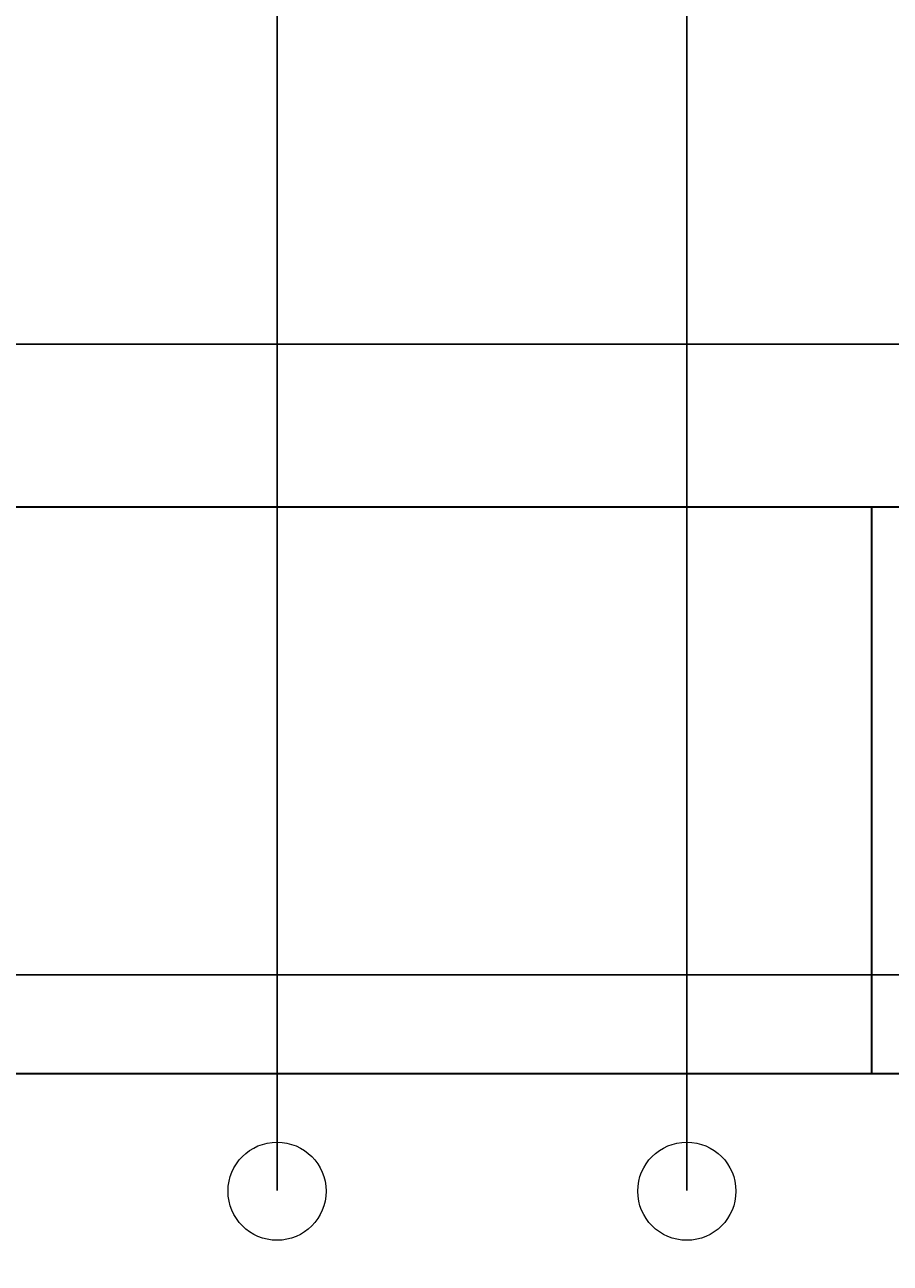
# Model space of a CAD drawing. Units: inches. Extents: x -13 to 809, y 112 to 656.
# Tile 30 of 55: x 183 to 257, y 446 to 551. Entities that reach past the tile are written whole.
import ezdxf

# ---------------------------------------------------------------- set-up
doc = ezdxf.new("R2010")
doc.units = ezdxf.units.IN
doc.header["$MEASUREMENT"] = 0
for name, color, linetype, lineweight in [('A-ANNO-DIMS', 2, 'Continuous', 18), ('A-ELEV', 7, 'Continuous', 35), ('A-ELEV-OTLN', 7, 'Continuous', 18)]:
    doc.layers.add(name, color=color, linetype=linetype, lineweight=lineweight)
doc.styles.get("Standard").update_dxf_attribs({"font": 'arial.ttf'})
doc.dimstyles.get("Standard").update_dxf_attribs({"dimtxt": 0.625, "dimasz": 0.18, "dimexe": 0.18, "dimexo": 0.0625, "dimgap": 0.09, "dimtad": 0, "dimtih": 1, "dimtoh": 1, "dimdec": 4, "dimzin": 0, "dimdsep": 46, "dimlunit": 4, "dimtxsty": 'Standard', "dimcen": 0.09, "dimadec": 0, "dimazin": 0, "dimtfac": 1, "dimtdec": 4, "dimtofl": 0, "dimtmove": 0, "dimatfit": 3, "dimfxl": 1, "dimtolj": 1, "dimtzin": 0, "dimarcsym": 0})

# ---------------------------------------------------------------- blocks, each defined once
blk = doc.blocks.new('*D23')
at = {"layer": 'A-ANNO-DIMS', "color": 0, "lineweight": -2, "transparency": 16777216}
for p, q in [((107.26, 510.58), (107.26, 655.96)), ((107.44, 655.78), (198.73, 655.78)), ((292.74, 655.78), (201.45, 655.78)), ((292.92, 569.3), (292.92, 655.96))]:
    blk.add_line(p, q, dxfattribs=at)
at = {"layer": 'A-ANNO-DIMS', "color": 0, "transparency": 16777216}
for points in [[(107.44, 655.81), (107.44, 655.75), (107.26, 655.78)], [(292.74, 655.81), (292.74, 655.75), (292.92, 655.78)]]:
    blk.add_solid(points, dxfattribs=at)
at = {"layer": 'Defpoints', "color": 0, "transparency": 16777216}
for p in [(292.92, 655.78), (292.92, 569.24), (107.26, 510.52)]:
    blk.add_point(p, dxfattribs=at)
at = {"layer": 'A-ANNO-DIMS', "color": 0, "transparency": 16777216, "insert": (200.09, 655.78), "char_height": 0.625, "attachment_point": 5}
blk.add_mtext('\\A1;185.66', dxfattribs=at)
blk = doc.blocks.new('*D36')
at = {"layer": 'A-ANNO-DIMS', "color": 0, "lineweight": -2, "transparency": 16777216}
for p, q in [((311.64, 569.24), (-12.1, 569.24)), ((-11.92, 569.06), (-11.92, 540.29)), ((-11.92, 510.7), (-11.92, 539.47)), ((107.2, 510.52), (-12.1, 510.52))]:
    blk.add_line(p, q, dxfattribs=at)
at = {"layer": 'A-ANNO-DIMS', "color": 0, "transparency": 16777216}
for points in [[(-11.95, 569.06), (-11.89, 569.06), (-11.92, 569.24)], [(-11.95, 510.7), (-11.89, 510.7), (-11.92, 510.52)]]:
    blk.add_solid(points, dxfattribs=at)
at = {"layer": 'Defpoints', "color": 0, "transparency": 16777216}
for p in [(-11.92, 569.24), (311.7, 569.24), (107.26, 510.52)]:
    blk.add_point(p, dxfattribs=at)
at = {"layer": 'A-ANNO-DIMS', "color": 0, "transparency": 16777216, "insert": (-11.92, 539.88), "char_height": 0.625, "attachment_point": 5}
blk.add_mtext('\\A1;58.72', dxfattribs=at)
blk = doc.blocks.new('*D39')
at = {"layer": 'A-ANNO-DIMS', "color": 0, "lineweight": -2, "transparency": 16777216}
for p, q in [((341.34, 524.28), (-12.1, 524.28)), ((-11.92, 524.1), (-11.92, 406.78)), ((-11.92, 288.63), (-11.92, 405.96)), ((341.34, 288.45), (-12.1, 288.45))]:
    blk.add_line(p, q, dxfattribs=at)
at = {"layer": 'A-ANNO-DIMS', "color": 0, "transparency": 16777216}
for points in [[(-11.95, 524.1), (-11.89, 524.1), (-11.92, 524.28)], [(-11.95, 288.63), (-11.89, 288.63), (-11.92, 288.45)]]:
    blk.add_solid(points, dxfattribs=at)
at = {"layer": 'Defpoints', "color": 0, "transparency": 16777216}
for p in [(-11.92, 524.28), (341.41, 524.28), (341.41, 288.45)]:
    blk.add_point(p, dxfattribs=at)
at = {"layer": 'A-ANNO-DIMS', "color": 0, "transparency": 16777216, "insert": (-11.92, 406.37), "char_height": 0.625, "attachment_point": 5}
blk.add_mtext('\\A1;235.83', dxfattribs=at)
blk = doc.blocks.new('*D43')
at = {"layer": 'A-ANNO-DIMS', "color": 0, "lineweight": -2, "transparency": 16777216}
for p, q in [((471.04, 470.88), (-12.1, 470.88)), ((-11.92, 470.7), (-11.92, 443.28)), ((-11.92, 415.04), (-11.92, 442.46)), ((471.04, 414.86), (-12.1, 414.86))]:
    blk.add_line(p, q, dxfattribs=at)
at = {"layer": 'A-ANNO-DIMS', "color": 0, "transparency": 16777216}
for points in [[(-11.95, 470.7), (-11.89, 470.7), (-11.92, 470.88)], [(-11.95, 415.04), (-11.89, 415.04), (-11.92, 414.86)]]:
    blk.add_solid(points, dxfattribs=at)
at = {"layer": 'Defpoints', "color": 0, "transparency": 16777216}
for p in [(-11.92, 470.88), (471.1, 470.88), (471.1, 414.86)]:
    blk.add_point(p, dxfattribs=at)
at = {"layer": 'A-ANNO-DIMS', "color": 0, "transparency": 16777216, "insert": (-11.92, 442.87), "char_height": 0.625, "attachment_point": 5}
blk.add_mtext('\\A1;56.02', dxfattribs=at)
blk = doc.blocks.new('*D98')
at = {"layer": 'A-ANNO-DIMS', "color": 0, "lineweight": -2, "transparency": 16777216}
for p, q in [((177.59, 452.63), (177.59, 655.96)), ((177.77, 655.78), (189.7, 655.78)), ((204.42, 655.78), (192.49, 655.78)), ((204.6, 452.63), (204.6, 655.96))]:
    blk.add_line(p, q, dxfattribs=at)
at = {"layer": 'A-ANNO-DIMS', "color": 0, "transparency": 16777216}
for points in [[(177.77, 655.81), (177.77, 655.75), (177.59, 655.78)], [(204.42, 655.81), (204.42, 655.75), (204.6, 655.78)]]:
    blk.add_solid(points, dxfattribs=at)
at = {"layer": 'Defpoints', "color": 0, "transparency": 16777216}
for p in [(204.6, 655.78), (177.59, 452.56), (204.6, 452.56)]:
    blk.add_point(p, dxfattribs=at)
at = {"layer": 'A-ANNO-DIMS', "color": 0, "transparency": 16777216, "insert": (191.09, 655.78), "char_height": 0.625, "attachment_point": 5}
blk.add_mtext('\\A1;27.017', dxfattribs=at)
blk = doc.blocks.new('*D99')
at = {"layer": 'A-ANNO-DIMS', "color": 0, "lineweight": -2, "transparency": 16777216}
for p, q in [((204.6, 452.63), (204.6, 655.96)), ((204.78, 655.78), (220.57, 655.78)), ((239.13, 655.78), (223.34, 655.78)), ((239.31, 452.63), (239.31, 655.96))]:
    blk.add_line(p, q, dxfattribs=at)
at = {"layer": 'A-ANNO-DIMS', "color": 0, "transparency": 16777216}
for points in [[(204.78, 655.81), (204.78, 655.75), (204.6, 655.78)], [(239.13, 655.81), (239.13, 655.75), (239.31, 655.78)]]:
    blk.add_solid(points, dxfattribs=at)
at = {"layer": 'Defpoints', "color": 0, "transparency": 16777216}
for p in [(239.31, 655.78), (204.6, 452.56), (239.31, 452.56)]:
    blk.add_point(p, dxfattribs=at)
at = {"layer": 'A-ANNO-DIMS', "color": 0, "transparency": 16777216, "insert": (221.96, 655.78), "char_height": 0.625, "attachment_point": 5}
blk.add_mtext('\\A1;34.705', dxfattribs=at)
blk = doc.blocks.new('*D100')
at = {"layer": 'A-ANNO-DIMS', "color": 0, "lineweight": -2, "transparency": 16777216}
for p, q in [((239.31, 452.63), (239.31, 655.96)), ((239.49, 655.78), (252.41, 655.78)), ((268.12, 655.78), (255.2, 655.78)), ((268.3, 452.63), (268.3, 655.96))]:
    blk.add_line(p, q, dxfattribs=at)
at = {"layer": 'A-ANNO-DIMS', "color": 0, "transparency": 16777216}
for points in [[(239.49, 655.81), (239.49, 655.75), (239.31, 655.78)], [(268.12, 655.81), (268.12, 655.75), (268.3, 655.78)]]:
    blk.add_solid(points, dxfattribs=at)
at = {"layer": 'Defpoints', "color": 0, "transparency": 16777216}
for p in [(268.3, 655.78), (239.31, 452.56), (268.3, 452.56)]:
    blk.add_point(p, dxfattribs=at)
at = {"layer": 'A-ANNO-DIMS', "color": 0, "transparency": 16777216, "insert": (253.8, 655.78), "char_height": 0.625, "attachment_point": 5}
blk.add_mtext('\\A1;28.994', dxfattribs=at)

msp = doc.modelspace()

# ---------------------------------------------------------------- linework, layer by layer
at = {"layer": 'A-ELEV'}
for p, q in [((107.2588, 510.5199), (341.4072, 510.5199)), ((254.968, 462.5199), (254.968, 510.5199)), ((95.0469, 462.5199), (337.5074, 462.5199))]:
    msp.add_line(p, q, dxfattribs=at)
at = {"layer": 'A-ELEV-OTLN'}
for centre in [(204.6029, 452.5629), (239.3079, 452.5629)]:
    msp.add_circle(centre, 4.1542, dxfattribs=at)

# ---------------------------------------------------------------- dimensions: what is measured, and where the dimension line sits
at = {"layer": 'A-ANNO-DIMS'}
for base, p1, p2, override, picture, middle in [((292.923, 655.7828), (107.2588, 510.5199), (292.923, 569.2414), {"dimdec": 2, "dimlfac": 1, "dimrnd": 0, "dimzin": 0, "dimdsep": 46, "dimlunit": 2}, '*D23', (200.0909, 655.7828)), ((204.6029, 655.7828), (177.5857, 452.5629), (204.6029, 452.5629), {"dimdec": 3, "dimlfac": 1, "dimrnd": 0, "dimzin": 0, "dimdsep": 46, "dimlunit": 2}, '*D98', (191.0943, 655.7828)), ((239.3079, 655.7828), (204.6029, 452.5629), (239.3079, 452.5629), {"dimdec": 3, "dimlfac": 1, "dimrnd": 0, "dimzin": 0, "dimdsep": 46, "dimlunit": 2}, '*D99', (221.9554, 655.7828)), ((268.3019, 655.7828), (239.3079, 452.5629), (268.3019, 452.5629), {"dimdec": 3, "dimlfac": 1, "dimrnd": 0, "dimzin": 0, "dimdsep": 46, "dimlunit": 2}, '*D100', (253.8049, 655.7828))]:
    dim = msp.add_linear_dim(base=base, p1=p1, p2=p2, dimstyle='Standard', override=override, dxfattribs=at)
    dim.commit()
    dim.dimension.update_dxf_attribs({"geometry": picture, "text_midpoint": middle})
for base, p1, p2, picture, middle in [((-11.9191, 569.2414), (107.2588, 510.5199), (311.6991, 569.2414), '*D36', (-11.9191, 539.8806)), ((-11.9191, 524.281), (341.4072, 288.4508), (341.4072, 524.281), '*D39', (-11.9191, 406.3659)), ((-11.9191, 470.8765), (471.0998, 414.8594), (471.0998, 470.8765), '*D43', (-11.9191, 442.8679))]:
    dim = msp.add_linear_dim(base=base, p1=p1, p2=p2, angle=90, dimstyle='Standard', override={"dimdec": 2, "dimlfac": 1, "dimrnd": 0, "dimzin": 0, "dimdsep": 46, "dimlunit": 2}, dxfattribs=at)
    dim.commit()
    dim.dimension.update_dxf_attribs({"geometry": picture, "text_midpoint": middle})

doc.saveas('drawing.dxf')
